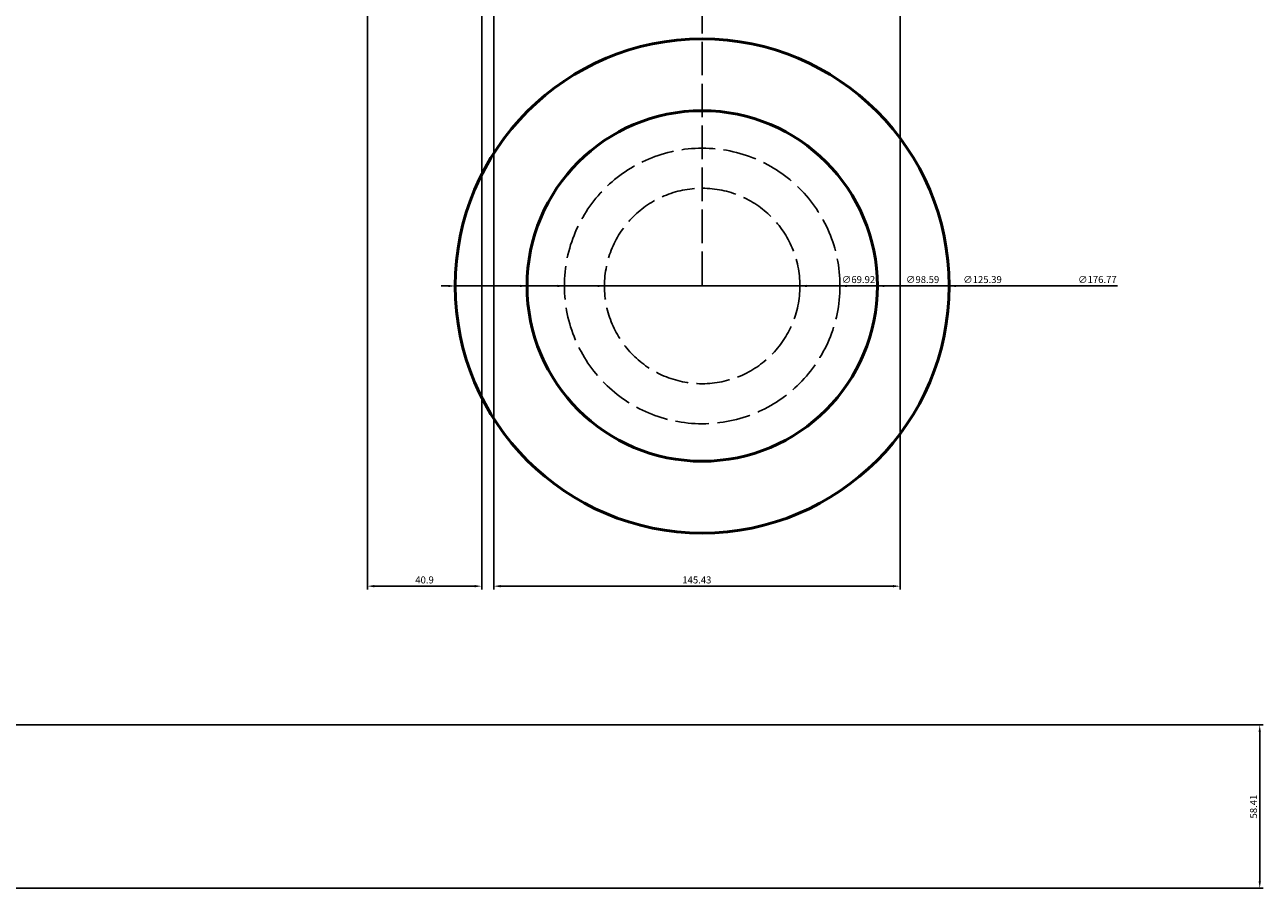
# Model space of a CAD drawing. Units: millimetres. Extents: x 921 to 2648, y 1390 to 2315.
# Tile 8 of 10: x 2205 to 2648, y 1411 to 1719. Entities that reach past the tile are written whole.
import ezdxf

# ---------------------------------------------------------------- set-up
doc = ezdxf.new("R2010")
doc.units = ezdxf.units.MM
doc.linetypes.add('ACAD_ISO02W100', pattern=[15, 12, -3])
for name, color, linetype, lineweight in [('M-DIMS', 2, 'Continuous', 25), ('M-HIDN', 4, 'ACAD_ISO02W100', 25), ('M-OUTL', 7, 'Continuous', 50)]:
    doc.layers.add(name, color=color, linetype=linetype, lineweight=lineweight)
doc.styles.get("Standard").update_dxf_attribs({"font": 'arial.ttf'})
doc.dimstyles.new('ISO-25', dxfattribs={"dimtxt": 2.5, "dimasz": 2.5, "dimexe": 1.25, "dimexo": 0.625, "dimtad": 1, "dimtxsty": 'Standard', "dimcen": 2.5, "dimadec": 0, "dimazin": 0, "dimtfac": 1, "dimtmove": 0, "dimatfit": 3, "dimfxl": 1, "dimarcsym": 0})

# ---------------------------------------------------------------- blocks, each defined once
blk = doc.blocks.new('*D40')
at = {"layer": 'Defpoints', "color": 0, "transparency": 16777216}
for p in [(2148.31, 1469), (2154.14, 1410.59), (2646.82, 1410.59)]:
    blk.add_point(p, dxfattribs=at)
at = {"layer": 'M-DIMS', "color": 0, "lineweight": -2, "transparency": 16777216}
for p, q in [((2148.94, 1469), (2648.07, 1469)), ((2646.82, 1466.5), (2646.82, 1413.09)), ((2154.77, 1410.59), (2648.07, 1410.59))]:
    blk.add_line(p, q, dxfattribs=at)
at = {"layer": 'M-DIMS', "color": 0, "transparency": 16777216}
for points in [[(2646.41, 1466.5), (2647.24, 1466.5), (2646.82, 1469)], [(2646.41, 1413.09), (2647.24, 1413.09), (2646.82, 1410.59)]]:
    blk.add_solid(points, dxfattribs=at)
at = {"layer": 'M-DIMS', "color": 0, "transparency": 16777216, "insert": (2644.92, 1439.79), "char_height": 2.5, "attachment_point": 5, "rotation": 90}
blk.add_mtext('58.41', dxfattribs=at)
blk = doc.blocks.new('*D95')
at = {"layer": 'Defpoints', "color": 0, "transparency": 16777216}
for p in [(2327.48, 1743.37), (2368.38, 1743.37), (2368.38, 1518.64)]:
    blk.add_point(p, dxfattribs=at)
at = {"layer": 'M-DIMS', "color": 0, "lineweight": -2, "transparency": 16777216}
for p, q in [((2327.48, 1742.75), (2327.48, 1517.39)), ((2368.38, 1742.75), (2368.38, 1517.39)), ((2329.98, 1518.64), (2365.88, 1518.64))]:
    blk.add_line(p, q, dxfattribs=at)
at = {"layer": 'M-DIMS', "color": 0, "transparency": 16777216}
for points in [[(2329.98, 1519.05), (2329.98, 1518.22), (2327.48, 1518.64)], [(2365.88, 1519.05), (2365.88, 1518.22), (2368.38, 1518.64)]]:
    blk.add_solid(points, dxfattribs=at)
at = {"layer": 'M-DIMS', "color": 0, "transparency": 16777216, "insert": (2347.93, 1520.54), "char_height": 2.5, "attachment_point": 5}
blk.add_mtext('40.9', dxfattribs=at)
blk = doc.blocks.new('*D96')
at = {"layer": 'Defpoints', "color": 0, "transparency": 16777216}
for p in [(2372.67, 1743.37), (2518.1, 1743.37), (2518.1, 1518.64)]:
    blk.add_point(p, dxfattribs=at)
at = {"layer": 'M-DIMS', "color": 0, "lineweight": -2, "transparency": 16777216}
for p, q in [((2372.67, 1742.75), (2372.67, 1517.39)), ((2518.1, 1742.75), (2518.1, 1517.39)), ((2375.17, 1518.64), (2515.6, 1518.64))]:
    blk.add_line(p, q, dxfattribs=at)
at = {"layer": 'M-DIMS', "color": 0, "transparency": 16777216}
for points in [[(2375.17, 1519.05), (2375.17, 1518.22), (2372.67, 1518.64)], [(2515.6, 1519.05), (2515.6, 1518.22), (2518.1, 1518.64)]]:
    blk.add_solid(points, dxfattribs=at)
at = {"layer": 'M-DIMS', "color": 0, "transparency": 16777216, "insert": (2445.38, 1520.54), "char_height": 2.5, "attachment_point": 5}
blk.add_mtext('145.43', dxfattribs=at)
blk = doc.blocks.new('*D106')
at = {"layer": 'Defpoints', "color": 0, "transparency": 16777216}
for p in [(2358.91, 1626.02), (2535.68, 1626.02)]:
    blk.add_point(p, dxfattribs=at)
at = {"layer": 'M-DIMS', "color": 0, "lineweight": -2, "transparency": 16777216}
for p, q in [((2356.41, 1626.02), (2353.91, 1626.02)), ((2358.91, 1626.02), (2535.68, 1626.02)), ((2595.88, 1626.02), (2538.18, 1626.02))]:
    blk.add_line(p, q, dxfattribs=at)
at = {"layer": 'M-DIMS', "color": 0, "transparency": 16777216}
for points in [[(2356.41, 1626.44), (2356.41, 1625.61), (2358.91, 1626.02)], [(2538.18, 1626.44), (2538.18, 1625.61), (2535.68, 1626.02)]]:
    blk.add_solid(points, dxfattribs=at)
at = {"layer": 'M-DIMS', "color": 0, "transparency": 16777216, "insert": (2588.71, 1627.99), "char_height": 2.5, "attachment_point": 5, "rotation": 0.0001}
blk.add_mtext('∅176.77', dxfattribs=at)
blk = doc.blocks.new('*D107')
at = {"layer": 'Defpoints', "color": 0, "transparency": 16777216}
for p in [(2384.6, 1626.02), (2509.99, 1626.02)]:
    blk.add_point(p, dxfattribs=at)
at = {"layer": 'M-DIMS', "color": 0, "lineweight": -2, "transparency": 16777216}
for p, q in [((2382.1, 1626.02), (2379.6, 1626.02)), ((2384.6, 1626.02), (2509.99, 1626.02)), ((2554.78, 1626.02), (2512.49, 1626.02))]:
    blk.add_line(p, q, dxfattribs=at)
at = {"layer": 'M-DIMS', "color": 0, "transparency": 16777216}
for points in [[(2382.1, 1626.44), (2382.1, 1625.61), (2384.6, 1626.02)], [(2512.49, 1626.44), (2512.49, 1625.61), (2509.99, 1626.02)]]:
    blk.add_solid(points, dxfattribs=at)
at = {"layer": 'M-DIMS', "color": 0, "transparency": 16777216, "insert": (2547.6, 1627.99), "char_height": 2.5, "attachment_point": 5, "rotation": 0.0002}
blk.add_mtext('∅125.39', dxfattribs=at)
blk = doc.blocks.new('*D108')
at = {"layer": 'Defpoints', "color": 0, "transparency": 16777216}
for p in [(2398, 1626.02), (2496.59, 1626.02)]:
    blk.add_point(p, dxfattribs=at)
at = {"layer": 'M-DIMS', "color": 0, "lineweight": -2, "transparency": 16777216}
for p, q in [((2395.5, 1626.02), (2393, 1626.02)), ((2398, 1626.02), (2496.59, 1626.02)), ((2532.37, 1626.02), (2499.09, 1626.02))]:
    blk.add_line(p, q, dxfattribs=at)
at = {"layer": 'M-DIMS', "color": 0, "transparency": 16777216}
for points in [[(2395.5, 1626.44), (2395.5, 1625.61), (2398, 1626.02)], [(2499.09, 1626.44), (2499.09, 1625.61), (2496.59, 1626.02)]]:
    blk.add_solid(points, dxfattribs=at)
at = {"layer": 'M-DIMS', "color": 0, "transparency": 16777216, "insert": (2526.16, 1627.99), "char_height": 2.5, "attachment_point": 5, "rotation": 0.0003}
blk.add_mtext('∅98.59', dxfattribs=at)
blk = doc.blocks.new('*D109')
at = {"layer": 'Defpoints', "color": 0, "transparency": 16777216}
for p in [(2412.33, 1626.02), (2482.25, 1626.02)]:
    blk.add_point(p, dxfattribs=at)
at = {"layer": 'M-DIMS', "color": 0, "lineweight": -2, "transparency": 16777216}
for p, q in [((2409.83, 1626.02), (2407.33, 1626.02)), ((2412.33, 1626.02), (2482.25, 1626.02)), ((2509.42, 1626.02), (2484.75, 1626.02))]:
    blk.add_line(p, q, dxfattribs=at)
at = {"layer": 'M-DIMS', "color": 0, "transparency": 16777216}
for points in [[(2409.83, 1626.44), (2409.83, 1625.61), (2412.33, 1626.02)], [(2484.75, 1626.44), (2484.75, 1625.61), (2482.25, 1626.02)]]:
    blk.add_solid(points, dxfattribs=at)
at = {"layer": 'M-DIMS', "color": 0, "transparency": 16777216, "insert": (2503.23, 1627.99), "char_height": 2.5, "attachment_point": 5, "rotation": 0.0004}
blk.add_mtext('∅69.92', dxfattribs=at)

msp = doc.modelspace()

# ---------------------------------------------------------------- linework, layer by layer
at = {"layer": 'M-HIDN'}
msp.add_line((2447.2926, 1743.373), (2447.2926, 1626.0228), dxfattribs=at)
for radius in [49.2928, 34.9614]:
    msp.add_circle((2447.2926, 1626.0228), radius, dxfattribs=at)
at = {"layer": 'M-OUTL'}
for radius in [88.3862, 88.3862, 88.3862, 62.6932]:
    msp.add_circle((2447.2926, 1626.0228), radius, dxfattribs=at)

# ---------------------------------------------------------------- dimensions: what is measured, and where the dimension line sits
at = {"layer": 'M-DIMS'}
for base, p1, p2, override, picture, middle in [((2368.3795, 1518.6366), (2327.4822, 1743.373), (2368.3795, 1743.373), {"dimdec": 1, "dimlfac": 1, "dimrnd": 0, "dimzin": 0, "dimdsep": 46, "dimlunit": 2}, '*D95', (2347.9309, 1520.538)), ((2518.0959, 1518.6366), (2372.6661, 1743.373), (2518.0959, 1743.373), {"dimdec": 2, "dimlfac": 1, "dimrnd": 0, "dimzin": 0, "dimdsep": 46, "dimlunit": 2}, '*D96', (2445.381, 1520.5389))]:
    dim = msp.add_linear_dim(base=base, p1=p1, p2=p2, dimstyle='ISO-25', override=override, dxfattribs=at)
    dim.commit()
    dim.dimension.update_dxf_attribs({"geometry": picture, "text_midpoint": middle})
for p1, p2, picture, middle in [((2358.9064, 1626.0225), (2535.6787, 1626.023), '*D106', (2588.7104, 1626.0231)), ((2384.5994, 1626.0225), (2509.9858, 1626.023), '*D107', (2547.6017, 1626.0231)), ((2397.9997, 1626.0225), (2496.5854, 1626.023), '*D108', (2526.1611, 1626.0231)), ((2412.3312, 1626.0225), (2482.2539, 1626.023), '*D109', (2503.2307, 1626.0231))]:
    dim = msp.add_diameter_dim_2p(p1=p1, p2=p2, dimstyle='ISO-25', override={"dimdec": 2, "dimlfac": 1, "dimrnd": 0, "dimzin": 0, "dimdsep": 46, "dimlunit": 2}, dxfattribs=at)
    dim.commit()
    dim.dimension.update_dxf_attribs({"geometry": picture, "text_midpoint": middle, "dimtype": 163})
dim = msp.add_linear_dim(base=(2646.8247, 1410.5877), p1=(2148.3108, 1468.998), p2=(2154.1446, 1410.5877), angle=90, dimstyle='ISO-25', override={"dimdec": 2, "dimlfac": 1, "dimrnd": 0, "dimzin": 0, "dimdsep": 46, "dimlunit": 2}, dxfattribs=at)
dim.commit()
dim.dimension.update_dxf_attribs({"geometry": '*D40', "text_midpoint": (2644.9233, 1439.7929)})

doc.saveas('drawing.dxf')
